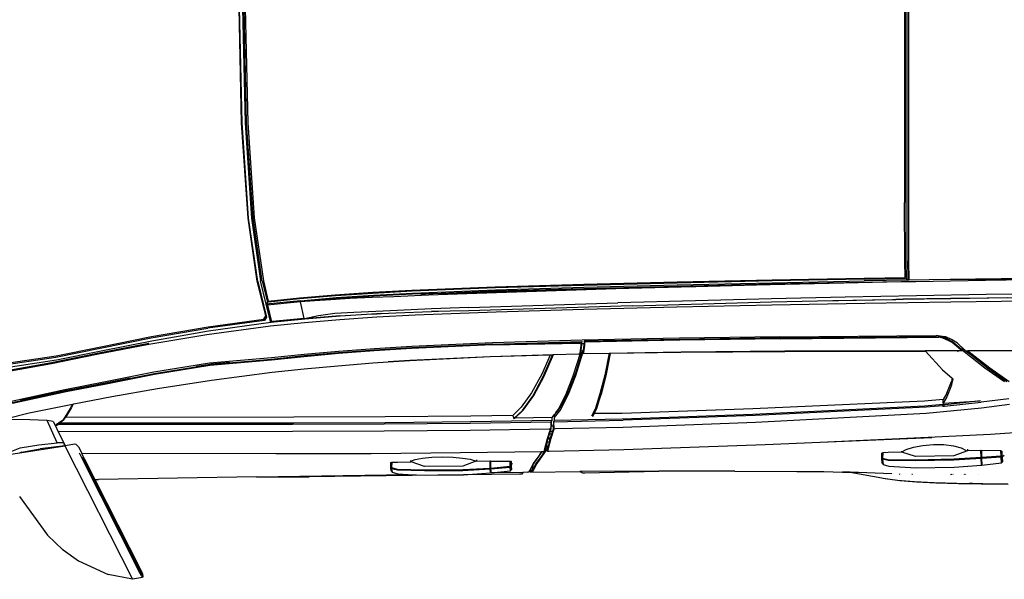
# Model space of a CAD drawing. Units: inches. Extents: x 22042254 to 25404563, y 17568978 to 17626777.
# Tile 14 of 45: x 22042341.458 to 22042342.604, y 17568977.553 to 17568978.204. Entities that reach past the tile are written whole.
import ezdxf

# ---------------------------------------------------------------- set-up
doc = ezdxf.new("R2010")
doc.units = ezdxf.units.IN
doc.header["$MEASUREMENT"] = 0
doc.layers.add('A-SITE-VEHI', color=8, linetype='Continuous', lineweight=18)
doc.layers.add('Edges', color=250, linetype='Continuous')

# ---------------------------------------------------------------- blocks, each defined once
blk = doc.blocks.new('Nissan Qashqai pl')
at = {"layer": 'Edges'}
for p, q in [((8.8918, 12.7444), (9.0186, 12.9956)), ((9.0186, 12.9956), (8.9731, 12.9865)), ((9.0374, 12.9925), (9.0186, 12.9956)), ((8.9173, 12.961), (8.9731, 12.9865)), ((9.0333, 12.9845), (8.9232, 12.7662)), ((9.0386, 12.9907), (8.9254, 12.7664)), ((8.9483, 12.8082), (9.0343, 12.9785)), ((9.0356, 12.9888), (9.0333, 12.9845)), ((9.0343, 12.9785), (9.0347, 12.9794)), ((9.0347, 12.9794), (9.0362, 12.9822)), ((9.0356, 12.9888), (9.0374, 12.9925)), ((9.0362, 12.9822), (9.037, 12.9838)), ((9.0371, 12.9841), (9.037, 12.9838)), ((9.0371, 12.9841), (9.0376, 12.985)), ((9.0376, 12.985), (9.0371, 12.9847)), ((9.0386, 12.9907), (9.0374, 12.9925)), ((9.0376, 12.985), (9.0386, 12.9907)), ((8.8885, 12.9405), (8.9173, 12.961)), ((8.8591, 12.9127), (8.8879, 12.94)), ((8.8885, 12.9405), (8.8879, 12.94)), ((8.8066, 12.84), (8.8591, 12.9127)), ((10.4573, 12.8093), (10.4889, 12.8119)), ((10.4613, 12.8099), (10.4926, 12.8125)), ((10.4889, 12.8119), (10.526, 12.8138)), ((10.4926, 12.8125), (10.5294, 12.8143)), ((10.526, 12.8138), (10.569, 12.8151)), ((10.5294, 12.8143), (10.5719, 12.8156)), ((10.569, 12.8151), (10.5919, 12.8155)), ((10.5719, 12.8156), (10.6176, 12.8164)), ((10.5919, 12.8155), (10.6151, 12.8159)), ((10.5981, 12.8157), (10.5919, 12.8155)), ((10.6174, 12.816), (10.5981, 12.8157)), ((10.6151, 12.8159), (10.6644, 12.8162)), ((10.6176, 12.8164), (10.6651, 12.8167)), ((8.928, 12.7679), (8.9483, 12.8082)), ((8.9483, 12.8082), (8.9552, 12.8081)), ((9.2517, 12.8031), (8.9552, 12.8081)), ((9.2517, 12.8031), (9.351, 12.803)), ((9.2517, 12.8031), (9.5372, 12.7983)), ((9.641, 12.7991), (9.351, 12.803)), ((9.5052, 12.7918), (9.5044, 12.7856)), ((9.5052, 12.7918), (9.5069, 12.7941)), ((9.5061, 12.7878), (9.5069, 12.7941)), ((9.5069, 12.7941), (9.5176, 12.7972)), ((9.5679, 12.792), (9.5168, 12.7904)), ((9.5176, 12.7972), (9.5372, 12.7983)), ((9.5372, 12.7983), (9.5689, 12.7999)), ((9.6401, 12.7914), (9.5679, 12.792)), ((9.5689, 12.7999), (9.641, 12.7991)), ((9.641, 12.7991), (9.6921, 12.7956)), ((9.7466, 12.7978), (9.641, 12.7991)), ((9.692, 12.7943), (9.6913, 12.7886)), ((9.6921, 12.7956), (9.692, 12.7943)), ((9.6922, 12.7943), (9.692, 12.7943)), ((9.6922, 12.7943), (9.6921, 12.7956)), ((9.7526, 12.7946), (9.6921, 12.7956)), ((9.6922, 12.7885), (9.693, 12.7955)), ((9.6922, 12.7885), (9.6922, 12.7943)), ((9.693, 12.7955), (9.7296, 12.7914)), ((9.7511, 12.7979), (9.7466, 12.7978)), ((9.7526, 12.7946), (9.7511, 12.7979)), ((9.7623, 12.7945), (9.7526, 12.7946)), ((9.7623, 12.7945), (9.7643, 12.7937)), ((9.7643, 12.7937), (9.7652, 12.7927)), ((9.7643, 12.7937), (9.7648, 12.7929)), ((9.7648, 12.7929), (9.7648, 12.7929)), ((9.7648, 12.7929), (9.7664, 12.7902)), ((9.7652, 12.7927), (9.7665, 12.7907)), ((9.7667, 12.7933), (9.7665, 12.7907)), ((9.7677, 12.7944), (9.7667, 12.7933)), ((9.7676, 12.7931), (9.7667, 12.7933)), ((9.7673, 12.7899), (9.7676, 12.7931)), ((9.769, 12.7926), (9.7676, 12.7931)), ((9.7677, 12.7944), (9.7677, 12.7944)), ((9.77, 12.7936), (9.7677, 12.7944)), ((9.7677, 12.7944), (9.8598, 12.7928)), ((9.7712, 12.7892), (9.769, 12.7926)), ((9.7734, 12.7884), (9.77, 12.7936)), ((9.8598, 12.7928), (9.8614, 12.7937)), ((9.8643, 12.7927), (9.8598, 12.7928)), ((9.8614, 12.7937), (9.8647, 12.7956)), ((10.0085, 12.7922), (9.8643, 12.7927)), ((9.8647, 12.7956), (9.869, 12.7954)), ((9.869, 12.7954), (10.0085, 12.7922)), ((10.0124, 12.7922), (10.0085, 12.7922)), ((10.1513, 12.7924), (10.0124, 12.7922)), ((10.1513, 12.7924), (10.2677, 12.793)), ((10.2677, 12.793), (10.3189, 12.7931)), ((10.3189, 12.7931), (10.3537, 12.7939)), ((10.3537, 12.7939), (10.3832, 12.7945)), ((10.3679, 12.7944), (10.3537, 12.7939)), ((10.3679, 12.7944), (10.4275, 12.8051)), ((10.4468, 12.7976), (10.3679, 12.7944)), ((10.4275, 12.8051), (10.4304, 12.8056)), ((10.4304, 12.8056), (10.4339, 12.8061)), ((10.4339, 12.8061), (10.4573, 12.8093)), ((10.4339, 12.8061), (10.4345, 12.8062)), ((10.4345, 12.8062), (10.4613, 12.8099)), ((10.4503, 12.7976), (10.4502, 12.7976)), ((10.4603, 12.7976), (10.4613, 12.7978)), ((10.4838, 12.7977), (10.4852, 12.7982)), ((10.5565, 12.7985), (10.5591, 12.7977)), ((10.5615, 12.7978), (10.5617, 12.7985)), ((10.583, 12.7984), (10.5834, 12.798)), ((10.5836, 12.798), (10.5831, 12.7984)), ((10.5847, 12.798), (10.5841, 12.7984)), ((10.5873, 12.7981), (10.5873, 12.7981)), ((10.6087, 12.7983), (10.6087, 12.7984)), ((9.5037, 12.7806), (9.5045, 12.7814)), ((9.5044, 12.7856), (9.5045, 12.7814)), ((9.5045, 12.7814), (9.5045, 12.7759)), ((9.5045, 12.7759), (9.5063, 12.7755)), ((9.5168, 12.7904), (9.5061, 12.7878)), ((9.5061, 12.7856), (9.5167, 12.7883)), ((9.5063, 12.7755), (9.5061, 12.7856)), ((9.5063, 12.7755), (9.5168, 12.7751)), ((9.5167, 12.7883), (9.5679, 12.7899)), ((9.5168, 12.7751), (9.5423, 12.7746)), ((9.5423, 12.7746), (9.5422, 12.7736)), ((9.5422, 12.7736), (9.5422, 12.7725)), ((9.5422, 12.7736), (9.5424, 12.7735)), ((9.5426, 12.7747), (9.5423, 12.7746)), ((9.5426, 12.7747), (9.5424, 12.7735)), ((9.5424, 12.7735), (9.5503, 12.7706)), ((9.5678, 12.7837), (9.5426, 12.7747)), ((9.64, 12.7831), (9.5678, 12.7837)), ((9.5679, 12.7899), (9.64, 12.7892)), ((9.64, 12.7892), (9.6912, 12.7865)), ((9.6645, 12.7737), (9.64, 12.7831)), ((9.6913, 12.7886), (9.6401, 12.7914)), ((9.6633, 12.7726), (9.6645, 12.7737)), ((9.6655, 12.7733), (9.6645, 12.7737)), ((9.6655, 12.7733), (9.6911, 12.7732)), ((9.6655, 12.7713), (9.6655, 12.7733)), ((9.6912, 12.7811), (9.6911, 12.7796)), ((9.6911, 12.7796), (9.6911, 12.7732)), ((9.6913, 12.7886), (9.6912, 12.7865)), ((9.6912, 12.7865), (9.6912, 12.7811)), ((9.692, 12.7811), (9.6912, 12.7811)), ((9.692, 12.7811), (9.6921, 12.7864)), ((9.692, 12.7796), (9.692, 12.7811)), ((9.692, 12.7733), (9.692, 12.7796)), ((9.692, 12.7733), (9.7287, 12.7734)), ((9.6922, 12.7885), (9.6921, 12.7864)), ((9.6921, 12.7864), (9.7288, 12.7832)), ((9.7288, 12.7854), (9.6922, 12.7885)), ((9.7288, 12.7832), (9.7287, 12.7734)), ((9.7287, 12.7734), (9.7305, 12.7738)), ((9.7296, 12.7914), (9.7288, 12.7854)), ((9.7306, 12.7834), (9.7288, 12.7854)), ((9.7288, 12.7854), (9.7288, 12.7832)), ((9.7288, 12.7832), (9.7306, 12.7834)), ((9.7296, 12.7914), (9.7314, 12.7895)), ((9.7305, 12.7738), (9.7306, 12.7834)), ((9.7305, 12.7738), (9.7313, 12.7798)), ((9.7306, 12.7834), (9.7314, 12.7895)), ((9.7314, 12.7895), (9.7313, 12.7798)), ((9.733, 12.7782), (9.7313, 12.7798)), ((9.7665, 12.7904), (9.7664, 12.7902)), ((9.7664, 12.7902), (9.7674, 12.7885)), ((9.7665, 12.7907), (9.7676, 12.7889)), ((9.7673, 12.7897), (9.7673, 12.7899)), ((9.7673, 12.7897), (9.7676, 12.7889)), ((9.7674, 12.7885), (9.7728, 12.7781)), ((9.7676, 12.7889), (9.7684, 12.7875)), ((9.7676, 12.7887), (9.7678, 12.7882)), ((9.7684, 12.7875), (9.7717, 12.781)), ((9.7707, 12.7848), (9.7709, 12.7893)), ((9.7717, 12.781), (9.7707, 12.7848)), ((9.7709, 12.7893), (9.7712, 12.7892)), ((9.7724, 12.7874), (9.7712, 12.7892)), ((9.7717, 12.781), (9.7738, 12.7771)), ((9.7778, 12.777), (9.7724, 12.7874)), ((9.7728, 12.7781), (9.7832, 12.7637)), ((9.7788, 12.778), (9.7734, 12.7884)), ((9.7738, 12.7771), (9.7842, 12.7627)), ((9.7883, 12.7626), (9.7778, 12.777)), ((9.7894, 12.7636), (9.7788, 12.778)), ((10.4282, 12.7775), (10.4274, 12.7679)), ((10.4282, 12.7775), (10.4299, 12.7798)), ((10.4291, 12.77), (10.4299, 12.7798)), ((10.4299, 12.7798), (10.4406, 12.7829)), ((10.4406, 12.7829), (10.4919, 12.7858)), ((10.4919, 12.7858), (10.564, 12.7851)), ((10.564, 12.7851), (10.6151, 12.7813)), ((10.615, 12.7803), (10.6142, 12.7686)), ((10.6151, 12.7813), (10.615, 12.7803)), ((10.615, 12.7676), (10.6151, 12.7803)), ((10.6151, 12.7803), (10.615, 12.7803)), ((10.6151, 12.7803), (10.6151, 12.7813)), ((10.6151, 12.7685), (10.616, 12.7812)), ((10.616, 12.7812), (10.6526, 12.7768)), ((10.6526, 12.7768), (10.6518, 12.7657)), ((10.6526, 12.7768), (10.6543, 12.7749)), ((10.6537, 12.7658), (10.6543, 12.7749)), ((10.6543, 12.7749), (10.6543, 12.7656)), ((8.7858, 12.7613), (8.807, 12.758)), ((8.8102, 12.7568), (8.807, 12.758)), ((8.807, 12.758), (8.8918, 12.7444)), ((8.8102, 12.7568), (8.8455, 12.7506)), ((8.9171, 12.7464), (8.9233, 12.7586)), ((8.9232, 12.7662), (8.9194, 12.7588)), ((8.925, 12.762), (8.9233, 12.7586)), ((8.9233, 12.7586), (9.2886, 12.7594)), ((8.928, 12.7679), (8.925, 12.762)), ((9.2886, 12.7594), (9.4673, 12.7589)), ((9.4673, 12.7589), (9.6358, 12.7575)), ((9.5503, 12.7706), (9.5641, 12.7681)), ((9.5641, 12.7681), (9.5818, 12.766)), ((9.5818, 12.766), (9.6016, 12.7651)), ((9.6016, 12.7651), (9.6215, 12.766)), ((9.6215, 12.766), (9.6395, 12.7676)), ((9.6358, 12.7575), (9.7887, 12.7552)), ((9.6395, 12.7676), (9.654, 12.7697)), ((9.654, 12.7697), (9.6633, 12.7726)), ((9.6911, 12.7732), (9.692, 12.7733)), ((9.7832, 12.7637), (9.7887, 12.7552)), ((9.7842, 12.7627), (9.7891, 12.7552)), ((9.7933, 12.7549), (9.7883, 12.7626)), ((9.7887, 12.7552), (9.7891, 12.7552)), ((9.7891, 12.7552), (9.79, 12.7552)), ((9.7965, 12.7526), (9.7894, 12.7636)), ((9.79, 12.7552), (9.7931, 12.7552)), ((9.7931, 12.7552), (9.7934, 12.7535)), ((9.7931, 12.7552), (9.7933, 12.7549)), ((9.7933, 12.7549), (9.7941, 12.7541)), ((9.7993, 12.755), (9.7986, 12.7544)), ((9.7999, 12.7522), (9.7993, 12.755)), ((9.7993, 12.755), (9.8024, 12.7549)), ((9.8024, 12.7549), (9.9426, 12.7518)), ((10.4263, 12.7665), (10.4274, 12.7674)), ((10.4274, 12.7679), (10.4274, 12.7674)), ((10.4274, 12.7674), (10.4275, 12.7586)), ((10.4293, 12.7579), (10.4275, 12.7586)), ((10.4398, 12.7724), (10.4291, 12.77)), ((10.4291, 12.7677), (10.4398, 12.7701)), ((10.4293, 12.7579), (10.4291, 12.7677)), ((10.4398, 12.7573), (10.4293, 12.7579)), ((10.4909, 12.773), (10.4398, 12.7724)), ((10.4398, 12.7701), (10.4909, 12.7708)), ((10.4653, 12.7564), (10.4398, 12.7573)), ((10.4653, 12.7561), (10.4652, 12.7545)), ((10.4908, 12.7648), (10.4653, 12.7564)), ((10.4653, 12.7564), (10.4653, 12.7561)), ((10.4653, 12.7564), (10.4653, 12.7564)), ((10.4653, 12.7564), (10.4653, 12.7561)), ((10.4653, 12.7561), (10.4653, 12.7561)), ((10.4653, 12.7561), (10.4732, 12.7517)), ((10.563, 12.7633), (10.4908, 12.7648)), ((10.5631, 12.7715), (10.4909, 12.773)), ((10.4909, 12.7708), (10.563, 12.7692)), ((10.563, 12.7692), (10.6142, 12.7663)), ((10.5867, 12.7545), (10.563, 12.7633)), ((10.6142, 12.7686), (10.5631, 12.7715)), ((10.6142, 12.766), (10.6141, 12.7537)), ((10.6142, 12.7686), (10.6142, 12.7677)), ((10.6142, 12.7677), (10.615, 12.7676)), ((10.6142, 12.7677), (10.6142, 12.7663)), ((10.6142, 12.7663), (10.6142, 12.766)), ((10.6151, 12.7676), (10.615, 12.7676)), ((10.615, 12.7537), (10.6151, 12.7659)), ((10.6518, 12.7657), (10.6151, 12.7685)), ((10.6151, 12.7676), (10.6151, 12.7685)), ((10.6151, 12.7662), (10.6151, 12.7676)), ((10.6151, 12.7662), (10.6518, 12.7634)), ((10.6151, 12.7659), (10.6151, 12.7662)), ((10.6518, 12.7634), (10.6517, 12.754)), ((10.6536, 12.7639), (10.6518, 12.7657)), ((10.6518, 12.7657), (10.6518, 12.7634)), ((10.6518, 12.7634), (10.6536, 12.7639)), ((10.6543, 12.7656), (10.6535, 12.7546)), ((10.6535, 12.7546), (10.6536, 12.7639)), ((10.6536, 12.7639), (10.6537, 12.7658)), ((10.6537, 12.7658), (10.6543, 12.7656)), ((10.6578, 12.7628), (10.6543, 12.7656)), ((8.7917, 12.7547), (8.8075, 12.7486)), ((8.8075, 12.7486), (8.8429, 12.7426)), ((8.8429, 12.7426), (8.8771, 12.7388)), ((8.8918, 12.7444), (8.8455, 12.7506)), ((8.8771, 12.7388), (8.8585, 12.6969)), ((8.8895, 12.7393), (8.8771, 12.7388)), ((8.8815, 12.7228), (8.892, 12.7444)), ((8.8815, 12.7228), (8.8895, 12.7393)), ((8.8908, 12.7421), (8.8895, 12.7393)), ((8.8906, 12.7418), (8.8895, 12.7393)), ((8.8906, 12.7418), (8.8911, 12.7428)), ((8.892, 12.7444), (8.8908, 12.7421)), ((8.8911, 12.7428), (8.8919, 12.7444)), ((8.8911, 12.7428), (8.8919, 12.7444)), ((8.8919, 12.7444), (8.8911, 12.7428)), ((8.8919, 12.7444), (8.8918, 12.7444)), ((8.892, 12.7444), (8.8919, 12.7444)), ((8.8919, 12.7444), (8.8919, 12.7444)), ((8.8919, 12.7444), (8.8919, 12.7444)), ((8.9106, 12.7413), (8.892, 12.7444)), ((8.892, 12.7444), (8.892, 12.7444)), ((8.9131, 12.7421), (8.9106, 12.7413)), ((8.9171, 12.7464), (8.9131, 12.7421)), ((8.9171, 12.7464), (8.917, 12.7468)), ((9.7934, 12.7535), (9.7938, 12.7538)), ((9.7934, 12.7535), (9.7937, 12.7524)), ((9.7937, 12.7524), (9.7992, 12.7308)), ((9.7941, 12.7541), (9.7943, 12.7535)), ((9.7955, 12.7516), (9.7943, 12.7535)), ((9.7943, 12.7535), (9.7964, 12.7453)), ((9.7963, 12.7523), (9.7955, 12.7516)), ((9.7963, 12.7523), (9.7963, 12.7524)), ((9.7964, 12.7524), (9.7963, 12.7523)), ((9.7992, 12.7476), (9.7963, 12.7523)), ((9.7967, 12.7526), (9.7964, 12.7524)), ((9.7964, 12.7525), (9.7964, 12.7524)), ((9.7964, 12.7524), (9.7996, 12.7475)), ((9.7964, 12.7453), (9.7992, 12.7476)), ((9.7964, 12.7453), (9.7973, 12.7418)), ((9.7983, 12.7541), (9.7965, 12.7526)), ((9.7965, 12.7526), (9.7967, 12.7526)), ((9.7977, 12.7535), (9.7967, 12.7526)), ((9.7967, 12.7526), (9.7986, 12.7526)), ((9.7977, 12.7431), (9.7973, 12.7418)), ((9.7973, 12.7418), (9.7977, 12.7409)), ((9.7973, 12.7418), (9.7977, 12.7399)), ((9.7982, 12.754), (9.7977, 12.7535)), ((9.7977, 12.7444), (9.7985, 12.7451)), ((9.7985, 12.7451), (9.7977, 12.7431)), ((9.7977, 12.7431), (9.7977, 12.7444)), ((9.7977, 12.7399), (9.7977, 12.7409)), ((9.7977, 12.7409), (9.7987, 12.7388)), ((9.7977, 12.7399), (9.7978, 12.7397)), ((9.7987, 12.7388), (9.7978, 12.7397)), ((9.7978, 12.7397), (9.7987, 12.7362)), ((9.7983, 12.7541), (9.7982, 12.754)), ((9.7986, 12.7526), (9.7982, 12.754)), ((9.7986, 12.7544), (9.7983, 12.7541)), ((9.7989, 12.7461), (9.7985, 12.7451)), ((9.7988, 12.7516), (9.7986, 12.7526)), ((9.7987, 12.7388), (9.7992, 12.7377)), ((9.7987, 12.7362), (9.7992, 12.7377)), ((9.7998, 12.7477), (9.7988, 12.7516)), ((9.7998, 12.7466), (9.7989, 12.7461)), ((9.7998, 12.7466), (9.7992, 12.7476)), ((9.7992, 12.7377), (9.8027, 12.7364)), ((9.7996, 12.7475), (9.7998, 12.7477)), ((9.8002, 12.7461), (9.7996, 12.7475)), ((9.8001, 12.7468), (9.7996, 12.7475)), ((9.8001, 12.7468), (9.7998, 12.7477)), ((9.8003, 12.7458), (9.7998, 12.7466)), ((9.8054, 12.7307), (9.7999, 12.7522)), ((9.8002, 12.7461), (9.8001, 12.7468)), ((9.8003, 12.7458), (9.8002, 12.7461)), ((9.8027, 12.7364), (9.8003, 12.7458)), ((9.8031, 12.7349), (9.8027, 12.7364)), ((9.9426, 12.7518), (10.2081, 12.7424)), ((10.2081, 12.7424), (10.312, 12.7377)), ((10.312, 12.7377), (10.5214, 12.7293)), ((10.312, 12.7377), (10.5147, 12.7285)), ((10.4732, 12.7517), (10.4871, 12.7474)), ((10.4871, 12.7474), (10.5048, 12.744)), ((10.5048, 12.744), (10.5246, 12.7423)), ((10.5246, 12.7423), (10.5445, 12.7425)), ((10.5445, 12.7425), (10.5625, 12.7446)), ((10.5625, 12.7446), (10.5769, 12.7484)), ((10.5769, 12.7484), (10.5863, 12.7537)), ((10.5863, 12.7537), (10.5867, 12.7545)), ((10.5885, 12.7538), (10.5867, 12.7545)), ((10.5885, 12.751), (10.5885, 12.7538)), ((10.6141, 12.7537), (10.5885, 12.7538)), ((10.6141, 12.7537), (10.615, 12.7537)), ((10.6517, 12.754), (10.615, 12.7537)), ((10.6535, 12.7546), (10.6517, 12.754)), ((8.8734, 12.7057), (8.8793, 12.7181)), ((8.8793, 12.7181), (8.8815, 12.7228)), ((9.3194, 12.7179), (8.8793, 12.7181)), ((9.4919, 12.7173), (9.3194, 12.7179)), ((9.7987, 12.7362), (9.8002, 12.7301)), ((9.7992, 12.7308), (9.8044, 12.7151)), ((9.8002, 12.7301), (9.8008, 12.7285)), ((9.8008, 12.7285), (9.8014, 12.7303)), ((9.8008, 12.7285), (9.8014, 12.7265)), ((9.8014, 12.7303), (9.8031, 12.7349)), ((9.8043, 12.7303), (9.8014, 12.7303)), ((9.8014, 12.7265), (9.803, 12.723)), ((9.8014, 12.7265), (9.8026, 12.723)), ((9.803, 12.723), (9.8026, 12.723)), ((9.8026, 12.723), (9.8046, 12.7171)), ((9.8067, 12.7229), (9.803, 12.723)), ((9.8043, 12.7303), (9.8031, 12.7349)), ((9.8044, 12.73), (9.8043, 12.7303)), ((9.8067, 12.7229), (9.8044, 12.73)), ((9.8106, 12.715), (9.8054, 12.7307)), ((9.8086, 12.7171), (9.8067, 12.7229)), ((10.5147, 12.7285), (10.6318, 12.7228)), ((10.6318, 12.7228), (10.6955, 12.7184)), ((8.87, 12.6987), (8.8734, 12.7057)), ((8.8734, 12.7057), (8.8768, 12.7057)), ((8.8751, 12.7054), (8.8768, 12.7057)), ((8.8893, 12.6956), (8.8751, 12.7054)), ((8.8768, 12.7057), (8.879, 12.704)), ((8.879, 12.704), (9.3198, 12.7039)), ((8.879, 12.704), (8.881, 12.7023)), ((9.3225, 12.7021), (8.881, 12.7023)), ((8.881, 12.7023), (8.8893, 12.6956)), ((9.3198, 12.7039), (9.4922, 12.7033)), ((9.4936, 12.7013), (9.3225, 12.7021)), ((9.6538, 12.7157), (9.4919, 12.7173)), ((9.4922, 12.7033), (9.654, 12.7018)), ((9.6552, 12.6997), (9.4936, 12.7013)), ((9.802, 12.7133), (9.6538, 12.7157)), ((9.654, 12.7018), (9.8061, 12.6994)), ((9.8078, 12.6971), (9.6552, 12.6997)), ((9.8051, 12.7132), (9.802, 12.7133)), ((9.8044, 12.7151), (9.8051, 12.7132)), ((9.8046, 12.7171), (9.8086, 12.7171)), ((9.8046, 12.7171), (9.8055, 12.7143)), ((9.8061, 12.6994), (9.8051, 12.7132)), ((9.8055, 12.7143), (9.8058, 12.7073)), ((9.8058, 12.7073), (9.8098, 12.7073)), ((9.8058, 12.7073), (9.8061, 12.6994)), ((9.8061, 12.6994), (9.8078, 12.6971)), ((9.8096, 12.7142), (9.8086, 12.7171)), ((9.8098, 12.7073), (9.8096, 12.7142)), ((9.8101, 12.6993), (9.8098, 12.7073)), ((9.8101, 12.6993), (9.8112, 12.7131)), ((9.8119, 12.697), (9.8101, 12.6993)), ((9.8101, 12.6993), (9.9411, 12.6966)), ((9.8112, 12.7131), (9.8106, 12.715)), ((9.8143, 12.713), (9.8112, 12.7131)), ((9.9414, 12.71), (9.8143, 12.713)), ((10.19, 12.7008), (9.9414, 12.71)), ((10.5113, 12.6839), (10.19, 12.7008)), ((8.7828, 12.6934), (8.8245, 12.6828)), ((8.8259, 12.6959), (8.7916, 12.6954)), ((8.8245, 12.6828), (8.9063, 12.6663)), ((8.8585, 12.6969), (8.8259, 12.6959)), ((8.87, 12.6987), (8.8585, 12.6969)), ((8.8893, 12.6956), (8.9021, 12.6745)), ((8.8913, 12.6936), (8.8893, 12.6956)), ((8.8927, 12.6913), (8.8913, 12.6936)), ((9.3224, 12.6911), (8.8927, 12.6913)), ((8.9041, 12.6725), (8.8927, 12.6913)), ((9.3225, 12.6911), (9.3224, 12.6911)), ((9.4936, 12.6904), (9.3225, 12.6911)), ((9.6552, 12.6888), (9.4936, 12.6904)), ((9.7337, 12.6875), (9.6552, 12.6888)), ((9.7337, 12.6875), (9.7357, 12.6935)), ((9.7499, 12.6721), (9.7337, 12.6875)), ((9.7357, 12.6935), (9.7378, 12.6924)), ((9.7357, 12.6935), (9.7519, 12.678)), ((9.7378, 12.6924), (9.754, 12.677)), ((9.8078, 12.6913), (9.7378, 12.6924)), ((9.8078, 12.6971), (9.8078, 12.6913)), ((9.8078, 12.6913), (9.8119, 12.6862)), ((9.9393, 12.6944), (9.8119, 12.697)), ((9.8119, 12.6912), (9.8119, 12.697)), ((9.8241, 12.6756), (9.8119, 12.6912)), ((9.8119, 12.6862), (9.8119, 12.6912)), ((9.8147, 12.6826), (9.8119, 12.6862)), ((9.8147, 12.6826), (9.8147, 12.6826)), ((9.8147, 12.6826), (9.8201, 12.6756)), ((9.8241, 12.6706), (9.8147, 12.6826)), ((9.8891, 12.6741), (9.8818, 12.6891)), ((9.8867, 12.6842), (9.8838, 12.6901)), ((9.9393, 12.684), (9.8867, 12.6842)), ((9.8911, 12.675), (9.8867, 12.6842)), ((10.1849, 12.6857), (9.9393, 12.6944)), ((10.1849, 12.6754), (9.9393, 12.684)), ((10.1894, 12.6879), (9.9411, 12.6966)), ((10.5079, 12.6703), (10.1849, 12.6857)), ((10.5109, 12.6721), (10.1894, 12.6879)), ((10.6152, 12.674), (10.5113, 12.6839)), ((8.8941, 12.6418), (8.7925, 12.664)), ((8.8942, 12.6432), (8.7931, 12.6653)), ((8.9021, 12.6745), (8.9063, 12.6663)), ((8.9075, 12.6661), (8.9041, 12.6725)), ((8.9063, 12.6663), (8.9075, 12.6661)), ((8.9075, 12.6661), (8.9087, 12.6658)), ((8.9087, 12.6658), (8.9797, 12.6518)), ((9.7692, 12.6453), (9.7499, 12.6721)), ((9.7519, 12.678), (9.7713, 12.6512)), ((9.754, 12.677), (9.7733, 12.6502)), ((9.8201, 12.6756), (9.8338, 12.6486)), ((9.8378, 12.6485), (9.8241, 12.6756)), ((9.8378, 12.6435), (9.8241, 12.6706)), ((9.8978, 12.6472), (9.8891, 12.6741)), ((9.8911, 12.6749), (9.8911, 12.675)), ((9.8931, 12.6691), (9.8911, 12.6749)), ((9.8911, 12.6749), (9.8998, 12.6481)), ((9.8931, 12.669), (9.8931, 12.6691)), ((9.8931, 12.669), (9.9018, 12.6421)), ((10.5079, 12.6607), (10.1849, 12.6754)), ((10.543, 12.6671), (10.5079, 12.6703)), ((10.5417, 12.6693), (10.5109, 12.6721)), ((10.5417, 12.6693), (10.5427, 12.6702)), ((10.5417, 12.6693), (10.543, 12.6671)), ((10.5436, 12.6687), (10.5427, 12.6702)), ((10.5427, 12.6702), (10.5458, 12.67)), ((10.544, 12.6678), (10.543, 12.6671)), ((10.543, 12.6646), (10.543, 12.6671)), ((10.543, 12.6646), (10.543, 12.6576)), ((10.5439, 12.6646), (10.543, 12.6646)), ((10.5502, 12.6526), (10.543, 12.6646)), ((10.544, 12.6678), (10.5436, 12.6687)), ((10.5439, 12.6646), (10.613, 12.6601)), ((10.547, 12.6674), (10.544, 12.6678)), ((10.5458, 12.67), (10.6144, 12.6629)), ((10.613, 12.6601), (10.547, 12.6674)), ((10.6664, 12.6566), (10.6144, 12.6629)), ((10.6678, 12.6672), (10.6152, 12.674)), ((8.8918, 12.6392), (8.7881, 12.6621)), ((8.8083, 12.6591), (8.8954, 12.6403)), ((8.9797, 12.6518), (9.0656, 12.6372)), ((9.7885, 12.6099), (9.7692, 12.6453)), ((9.7713, 12.6512), (9.7905, 12.6158)), ((9.7733, 12.6502), (9.7925, 12.6148)), ((9.8338, 12.6486), (9.8475, 12.613)), ((9.8516, 12.6129), (9.8378, 12.6485)), ((9.9066, 12.6119), (9.8978, 12.6472)), ((9.9086, 12.6129), (9.8998, 12.6481)), ((10.543, 12.6576), (10.5079, 12.6607)), ((10.5502, 12.6456), (10.543, 12.6576)), ((10.5584, 12.6306), (10.5502, 12.6526)), ((10.5502, 12.6456), (10.5584, 12.6236)), ((8.9679, 12.6241), (8.8918, 12.6392)), ((9.0601, 12.6092), (8.8941, 12.6418)), ((8.9696, 12.6285), (8.8942, 12.6432)), ((8.8961, 12.6401), (8.9704, 12.6257)), ((9.06, 12.6106), (8.9696, 12.6285)), ((8.9704, 12.6257), (8.9708, 12.6256)), ((8.9708, 12.6256), (9.0143, 12.6169)), ((9.0656, 12.6372), (9.1676, 12.6212)), ((9.8516, 12.6079), (9.8378, 12.6435)), ((9.9018, 12.6421), (9.9106, 12.6068)), ((10.5584, 12.6306), (10.5617, 12.619)), ((8.8666, 12.5888), (8.7287, 12.6134)), ((8.7292, 12.6146), (8.8666, 12.5901)), ((9.0591, 12.6065), (8.9679, 12.6241)), ((9.1644, 12.5938), (9.06, 12.6106)), ((9.1645, 12.5924), (9.0601, 12.6092)), ((9.1676, 12.6212), (9.2814, 12.6065)), ((9.8039, 12.5741), (9.7885, 12.6099)), ((9.7905, 12.6158), (9.8087, 12.574)), ((9.7925, 12.6148), (9.8107, 12.573)), ((9.8475, 12.613), (9.8611, 12.5708)), ((9.8652, 12.5704), (9.8516, 12.6129)), ((9.8652, 12.5654), (9.8516, 12.6079)), ((9.9149, 12.5705), (9.9066, 12.6119)), ((9.9169, 12.5714), (9.9086, 12.6129)), ((9.9106, 12.6068), (9.9177, 12.5714)), ((10.5419, 12.6018), (10.56, 12.6176)), ((10.56, 12.6176), (10.5584, 12.6236)), ((10.56, 12.6176), (10.5617, 12.619)), ((10.6583, 12.6245), (10.6215, 12.5986)), ((10.6627, 12.6241), (10.6261, 12.5984)), ((10.6306, 12.5982), (10.6671, 12.6238)), ((8.7481, 12.5968), (8.8745, 12.5782)), ((8.7491, 12.594), (8.8754, 12.5755)), ((8.8761, 12.5839), (8.7496, 12.6025)), ((8.8666, 12.5901), (8.9521, 12.5726)), ((8.9522, 12.5713), (8.8666, 12.5888)), ((9.1639, 12.5895), (9.0591, 12.6065)), ((9.1393, 12.5951), (9.1647, 12.591)), ((9.2801, 12.5794), (9.1639, 12.5895)), ((9.2803, 12.5836), (9.1644, 12.5938)), ((9.2804, 12.5821), (9.1645, 12.5924)), ((9.1647, 12.591), (9.1668, 12.5908)), ((9.1668, 12.5908), (9.2019, 12.5877)), ((9.2814, 12.6065), (9.3416, 12.5999)), ((9.3416, 12.5999), (9.4048, 12.5941)), ((9.4048, 12.5941), (9.471, 12.5888)), ((9.471, 12.5888), (9.4997, 12.5869)), ((10.51, 12.5666), (10.5419, 12.6018)), ((10.6215, 12.5986), (10.5796, 12.5655)), ((10.5892, 12.5659), (10.6306, 12.5982)), ((10.6261, 12.5984), (10.593, 12.5726)), ((8.8745, 12.5782), (8.9583, 12.5609)), ((8.8754, 12.5755), (8.9591, 12.5583)), ((8.9598, 12.5666), (8.8761, 12.5839)), ((8.9521, 12.5726), (9.0495, 12.5536)), ((9.0497, 12.5523), (8.9522, 12.5713)), ((9.3418, 12.5729), (9.2801, 12.5794)), ((9.3418, 12.5771), (9.2803, 12.5836)), ((9.3419, 12.5756), (9.2804, 12.5821)), ((9.4062, 12.5713), (9.3418, 12.5771)), ((9.4064, 12.5671), (9.3418, 12.5729)), ((9.4063, 12.5699), (9.3419, 12.5756)), ((9.4735, 12.5663), (9.4062, 12.5713)), ((9.4736, 12.5648), (9.4063, 12.5699)), ((9.5404, 12.5844), (9.4997, 12.5869)), ((9.4997, 12.5869), (9.5403, 12.5842)), ((9.5403, 12.5842), (9.6913, 12.5767)), ((9.6912, 12.5774), (9.5404, 12.5844)), ((9.8039, 12.5741), (9.6912, 12.5774)), ((9.6913, 12.5767), (9.8099, 12.573)), ((9.8087, 12.574), (9.8039, 12.5741)), ((9.8099, 12.573), (9.8087, 12.574)), ((9.8099, 12.573), (9.8107, 12.573)), ((9.8107, 12.573), (9.8573, 12.5716)), ((9.8573, 12.5716), (9.8603, 12.5715)), ((9.8603, 12.5715), (9.8605, 12.5696)), ((9.8611, 12.5708), (9.8603, 12.5715)), ((9.8612, 12.5707), (9.8611, 12.5708)), ((9.8612, 12.5707), (9.8615, 12.5688)), ((9.8652, 12.5706), (9.8664, 12.5714)), ((9.8652, 12.5706), (9.8665, 12.5695)), ((9.8652, 12.5704), (9.8652, 12.5706)), ((9.8652, 12.5704), (9.8652, 12.5704)), ((9.8652, 12.5704), (9.8652, 12.5654)), ((9.8655, 12.5687), (9.8652, 12.5704)), ((9.8665, 12.5695), (9.8664, 12.5714)), ((9.8664, 12.5714), (9.9149, 12.5705)), ((9.9149, 12.5705), (10.0505, 12.5681)), ((9.9177, 12.5714), (9.9169, 12.5714)), ((10.0501, 12.5695), (9.9177, 12.5714)), ((10.593, 12.5726), (10.584, 12.5655)), ((8.9583, 12.5609), (9.0538, 12.5419)), ((8.9591, 12.5583), (9.0546, 12.5394)), ((9.0552, 12.5477), (8.9598, 12.5666)), ((9.0495, 12.5536), (9.1584, 12.5351)), ((9.4739, 12.5621), (9.4064, 12.5671)), ((9.5437, 12.5619), (9.4735, 12.5663)), ((9.5438, 12.5605), (9.4736, 12.5648)), ((9.5443, 12.5579), (9.4739, 12.5621)), ((9.6953, 12.5549), (9.5437, 12.5619)), ((9.6954, 12.5535), (9.5438, 12.5605)), ((9.696, 12.551), (9.5443, 12.5579)), ((9.6953, 12.5549), (9.8598, 12.5517)), ((9.6953, 12.5549), (9.863, 12.5497)), ((9.6954, 12.5535), (9.8641, 12.5483)), ((9.8629, 12.5516), (9.8598, 12.5517)), ((9.8605, 12.5696), (9.8626, 12.5564)), ((9.8615, 12.5688), (9.8635, 12.5556)), ((9.8626, 12.5564), (9.8627, 12.5532)), ((9.8637, 12.5532), (9.8627, 12.5532)), ((9.8627, 12.5532), (9.8629, 12.5516)), ((9.8629, 12.5516), (9.863, 12.5497)), ((9.8635, 12.5556), (9.8637, 12.5532)), ((9.8643, 12.5532), (9.8637, 12.5532)), ((9.8637, 12.5532), (9.8638, 12.5508)), ((9.8677, 12.5531), (9.8643, 12.5532)), ((9.8675, 12.5555), (9.8655, 12.5687)), ((9.8686, 12.5562), (9.8665, 12.5695)), ((9.8677, 12.5531), (9.8675, 12.5555)), ((9.8678, 12.5507), (9.8677, 12.5531)), ((9.8689, 12.5515), (9.8686, 12.5562)), ((9.869, 12.5496), (9.8689, 12.5515)), ((10.2453, 12.568), (10.0501, 12.5695)), ((10.0505, 12.5681), (10.2453, 12.5664)), ((10.4292, 12.5674), (10.2453, 12.568)), ((10.2453, 12.5664), (10.4289, 12.5658)), ((10.4289, 12.5658), (10.5092, 12.5658)), ((10.5099, 12.5674), (10.4292, 12.5674)), ((10.5099, 12.5674), (10.5092, 12.5658)), ((10.5092, 12.5658), (10.5094, 12.5658)), ((10.5094, 12.5658), (10.51, 12.5666)), ((10.5783, 12.5659), (10.5094, 12.5658)), ((10.51, 12.5666), (10.5099, 12.5674)), ((10.57, 12.5517), (10.5589, 12.5451)), ((10.5764, 12.5642), (10.5598, 12.5507)), ((10.5776, 12.5633), (10.5612, 12.5498)), ((10.5834, 12.5641), (10.57, 12.5517)), ((10.57, 12.5517), (10.5821, 12.5633)), ((10.5709, 12.5675), (10.5705, 12.5671)), ((10.5719, 12.5682), (10.5709, 12.5675)), ((10.5783, 12.5659), (10.5764, 12.5642)), ((10.5776, 12.5633), (10.5783, 12.5659)), ((10.5796, 12.5655), (10.5776, 12.5633)), ((10.5796, 12.5655), (10.5783, 12.5659)), ((10.5796, 12.562), (10.5796, 12.5655)), ((10.5838, 12.5653), (10.5821, 12.5633)), ((10.584, 12.5647), (10.5834, 12.5641)), ((10.584, 12.5655), (10.5838, 12.5653)), ((10.584, 12.5655), (10.5841, 12.5655)), ((10.584, 12.5654), (10.584, 12.5655)), ((10.5847, 12.5655), (10.584, 12.5647)), ((10.584, 12.5647), (10.584, 12.5654)), ((10.5851, 12.5659), (10.5841, 12.5655)), ((10.5841, 12.5655), (10.5847, 12.5655)), ((10.5851, 12.5659), (10.5847, 12.5655)), ((10.5851, 12.5659), (10.5892, 12.5659)), ((10.6988, 12.5662), (10.5892, 12.5659)), ((9.0538, 12.5419), (9.1605, 12.5233)), ((9.0546, 12.5394), (9.1612, 12.5208)), ((9.1617, 12.5292), (9.0552, 12.5477)), ((9.1584, 12.5351), (9.2783, 12.5191)), ((9.8644, 12.5459), (9.696, 12.551)), ((9.8641, 12.5483), (9.863, 12.5497)), ((9.8638, 12.5508), (9.8641, 12.5483)), ((10.0472, 12.5423), (9.8644, 12.5459)), ((9.8681, 12.5482), (9.8678, 12.5507)), ((9.8681, 12.5482), (9.869, 12.5496)), ((10.0476, 12.5445), (9.8681, 12.5482)), ((10.0477, 12.5459), (9.869, 12.5496)), ((10.2357, 12.5398), (10.0472, 12.5423)), ((10.2367, 12.5419), (10.0476, 12.5445)), ((10.2369, 12.5433), (10.0477, 12.5459)), ((10.2357, 12.5398), (10.53, 12.5373)), ((10.2367, 12.5419), (10.5351, 12.5392)), ((10.2369, 12.5433), (10.5348, 12.5406)), ((10.4153, 12.5384), (10.4176, 12.5384)), ((10.4176, 12.5384), (10.4181, 12.5384)), ((10.4181, 12.5384), (10.4552, 12.538)), ((10.4181, 12.5384), (10.4181, 12.5384)), ((10.4778, 12.5378), (10.53, 12.5373)), ((10.5301, 12.5373), (10.53, 12.5373)), ((10.5335, 12.5378), (10.5301, 12.5373)), ((10.5419, 12.5391), (10.5335, 12.5378)), ((10.5422, 12.542), (10.5348, 12.5406)), ((10.5418, 12.5405), (10.5351, 12.5392)), ((10.5424, 12.5406), (10.5418, 12.5405)), ((10.5419, 12.5391), (10.5463, 12.541)), ((10.5479, 12.54), (10.5419, 12.5391)), ((10.5522, 12.5465), (10.5422, 12.542)), ((10.5495, 12.5438), (10.5424, 12.5406)), ((10.5463, 12.541), (10.5551, 12.5457)), ((10.5589, 12.5451), (10.5479, 12.54)), ((10.5546, 12.546), (10.5495, 12.5438)), ((10.5598, 12.5507), (10.5522, 12.5465)), ((10.5583, 12.5481), (10.5546, 12.546)), ((10.5551, 12.5457), (10.5583, 12.5481)), ((10.5612, 12.5498), (10.5583, 12.5481)), ((9.2669, 12.5088), (9.1605, 12.5233)), ((9.1612, 12.5208), (9.2656, 12.5065)), ((9.2789, 12.5131), (9.1617, 12.5292)), ((9.2783, 12.5191), (9.3422, 12.5126)), ((9.2694, 12.5006), (9.2535, 12.4354)), ((9.2543, 12.4356), (9.2707, 12.5028)), ((9.2656, 12.5065), (9.2669, 12.5088)), ((9.2656, 12.5065), (9.2694, 12.5006)), ((9.2707, 12.5028), (9.2669, 12.5088)), ((9.2707, 12.5028), (9.2694, 12.5006)), ((9.2789, 12.5131), (9.2704, 12.4783)), ((9.2724, 12.4804), (9.2799, 12.5114)), ((9.2799, 12.5114), (9.2789, 12.5131)), ((9.3427, 12.5066), (9.2789, 12.5131)), ((9.2819, 12.5112), (9.2799, 12.5114)), ((9.2803, 12.5116), (9.2822, 12.5118)), ((9.3418, 12.5051), (9.2819, 12.5112)), ((9.3418, 12.5051), (9.3346, 12.4741)), ((9.342, 12.5059), (9.3418, 12.5051)), ((9.3687, 12.5), (9.342, 12.5059)), ((9.4087, 12.5003), (9.342, 12.5059)), ((9.3422, 12.5126), (9.4088, 12.507)), ((9.4093, 12.5011), (9.3427, 12.5066)), ((9.3992, 12.496), (9.3687, 12.5)), ((9.4347, 12.494), (9.3992, 12.496)), ((9.4087, 12.5003), (9.4688, 12.4968)), ((9.4088, 12.507), (9.4782, 12.5024)), ((9.4785, 12.4965), (9.4093, 12.5011)), ((9.4688, 12.4968), (9.4789, 12.4964)), ((9.4782, 12.5024), (9.5503, 12.4987)), ((9.4789, 12.4964), (9.4785, 12.4965)), ((9.4862, 12.4961), (9.4785, 12.4965)), ((9.4789, 12.4964), (9.4862, 12.4961)), ((9.4862, 12.4961), (9.514, 12.4949)), ((9.5503, 12.4987), (9.7029, 12.4926)), ((9.2704, 12.4783), (9.2598, 12.4348)), ((9.2724, 12.4804), (9.2704, 12.4783)), ((9.2726, 12.4746), (9.2704, 12.4783)), ((9.3346, 12.4718), (9.2704, 12.4783)), ((9.3346, 12.4741), (9.2724, 12.4804)), ((9.4761, 12.4919), (9.4347, 12.494)), ((9.5168, 12.4903), (9.4761, 12.4919)), ((9.514, 12.4949), (9.5811, 12.492)), ((9.5812, 12.4874), (9.5168, 12.4903)), ((9.651, 12.4906), (9.5811, 12.492)), ((9.5811, 12.492), (9.594, 12.4914)), ((9.6514, 12.4849), (9.5812, 12.4874)), ((9.9583, 12.4812), (9.651, 12.4906)), ((9.6514, 12.4849), (9.9312, 12.4761)), ((9.7029, 12.4926), (9.8673, 12.4878)), ((9.8673, 12.4878), (10.0423, 12.4835)), ((9.9583, 12.4812), (10.091, 12.4775)), ((10.0423, 12.4835), (10.2211, 12.4795)), ((10.091, 12.4775), (10.2202, 12.4743)), ((10.2211, 12.4795), (10.3955, 12.4762)), ((9.2629, 12.435), (9.2726, 12.4746)), ((9.2649, 12.4348), (9.2741, 12.4725)), ((9.2746, 12.4744), (9.2726, 12.4746)), ((9.2741, 12.4725), (9.3326, 12.4666)), ((9.333, 12.4685), (9.2746, 12.4744)), ((9.3326, 12.4666), (9.4, 12.4609)), ((9.4004, 12.4629), (9.333, 12.4685)), ((9.3346, 12.4741), (9.3344, 12.4733)), ((9.3344, 12.4733), (9.4017, 12.4677)), ((9.3344, 12.4733), (9.3611, 12.4715)), ((9.3346, 12.4718), (9.4018, 12.4661)), ((9.3611, 12.4715), (9.3918, 12.4695)), ((9.3918, 12.4695), (9.4276, 12.4674)), ((9.4, 12.4609), (9.4706, 12.4561)), ((9.4709, 12.4581), (9.4004, 12.4629)), ((9.4017, 12.4677), (9.472, 12.463)), ((9.4018, 12.4661), (9.472, 12.4614)), ((9.4276, 12.4674), (9.4694, 12.4654)), ((9.4694, 12.4654), (9.5105, 12.4637)), ((9.472, 12.463), (9.5454, 12.4591)), ((9.472, 12.4614), (9.5454, 12.4576)), ((9.5105, 12.4637), (9.5755, 12.4608)), ((9.5454, 12.4591), (9.5454, 12.4593)), ((9.5695, 12.4589), (9.5454, 12.4591)), ((9.5609, 12.4593), (9.5695, 12.4589)), ((9.5786, 12.4588), (9.5695, 12.4589)), ((9.5695, 12.4589), (9.7014, 12.4536)), ((9.5755, 12.4608), (9.6472, 12.4581)), ((9.6206, 12.4581), (9.5786, 12.4588)), ((10.0776, 12.4719), (9.9312, 12.4761)), ((10.2201, 12.4683), (10.0776, 12.4719)), ((10.3586, 12.4651), (10.2201, 12.4683)), ((10.2202, 12.4743), (10.2203, 12.4743)), ((10.2203, 12.4743), (10.3353, 12.4717)), ((10.3353, 12.4717), (10.4477, 12.4694)), ((10.3353, 12.4717), (10.346, 12.4714)), ((10.346, 12.4714), (10.4477, 12.4694)), ((10.4931, 12.4624), (10.3586, 12.4651)), ((10.3955, 12.4762), (10.5572, 12.4737)), ((10.4477, 12.4694), (10.4538, 12.4693)), ((10.4538, 12.4693), (10.4681, 12.469)), ((10.4676, 12.4691), (10.4538, 12.4693)), ((10.5566, 12.4677), (10.4676, 12.4691)), ((10.4676, 12.4691), (10.546, 12.4677)), ((10.4681, 12.469), (10.5866, 12.467)), ((10.6237, 12.4603), (10.4931, 12.4624)), ((10.546, 12.4677), (10.546, 12.4678)), ((10.546, 12.4677), (10.5576, 12.4675)), ((10.7, 12.4662), (10.5566, 12.4677)), ((10.5572, 12.4737), (10.7004, 12.4722)), ((10.5576, 12.4675), (10.6649, 12.4659)), ((10.5866, 12.467), (10.6649, 12.4659)), ((10.7502, 12.4586), (10.6237, 12.4603)), ((9.4706, 12.4561), (9.5443, 12.4522)), ((9.5446, 12.4542), (9.4709, 12.4581)), ((9.5443, 12.4522), (9.701, 12.4459)), ((9.7011, 12.4478), (9.5446, 12.4542)), ((9.5454, 12.4576), (9.7014, 12.4513)), ((9.6714, 12.4567), (9.6206, 12.4581)), ((9.6414, 12.458), (9.6407, 12.458)), ((9.6472, 12.4581), (9.9278, 12.4492)), ((9.6549, 12.4576), (9.6558, 12.4574)), ((9.6825, 12.4564), (9.6714, 12.4567)), ((9.6825, 12.4564), (9.6829, 12.4563)), ((9.6943, 12.456), (9.6825, 12.4564)), ((9.6943, 12.4558), (9.6943, 12.456)), ((9.6951, 12.456), (9.6943, 12.456)), ((9.6951, 12.4558), (9.6951, 12.456)), ((9.8565, 12.451), (9.6951, 12.456)), ((9.701, 12.4459), (9.8673, 12.441)), ((9.8673, 12.443), (9.7011, 12.4478)), ((9.7014, 12.4536), (9.8673, 12.4488)), ((9.7014, 12.4513), (9.8673, 12.4464)), ((9.9794, 12.4475), (9.8565, 12.451)), ((9.8673, 12.4488), (10.0429, 12.4444)), ((9.8673, 12.4464), (10.0429, 12.4421)), ((10.043, 12.4387), (9.8673, 12.443)), ((9.8673, 12.441), (10.0431, 12.4367)), ((9.9278, 12.4492), (10.0747, 12.445)), ((10.0998, 12.4443), (9.9794, 12.4475)), ((10.0429, 12.4444), (10.2216, 12.4404)), ((10.0429, 12.4421), (10.2215, 12.4381)), ((10.0747, 12.445), (10.078, 12.4449)), ((10.078, 12.4449), (10.2146, 12.4414)), ((10.2146, 12.4414), (10.0998, 12.4443)), ((10.2146, 12.4414), (10.2175, 12.4413)), ((10.2175, 12.4413), (10.3564, 12.4382)), ((10.2216, 12.4404), (10.3947, 12.4371)), ((9.2535, 12.4354), (9.2362, 12.3167)), ((9.2543, 12.4356), (9.2371, 12.3169)), ((9.2426, 12.3164), (9.2598, 12.4348)), ((9.2629, 12.435), (9.2457, 12.3164)), ((9.2476, 12.3163), (9.2649, 12.4348)), ((10.2218, 12.4347), (10.043, 12.4387)), ((10.0431, 12.4367), (10.2218, 12.4327)), ((10.2215, 12.4381), (10.3945, 12.4348)), ((10.3947, 12.4314), (10.2218, 12.4347)), ((10.2218, 12.4327), (10.3947, 12.4294)), ((10.3564, 12.4382), (10.4638, 12.436)), ((10.4773, 12.4335), (10.3945, 12.4348)), ((10.3947, 12.4371), (10.4638, 12.436)), ((10.3947, 12.4314), (10.4735, 12.4301)), ((10.3947, 12.4294), (10.4715, 12.4282)), ((10.4638, 12.436), (10.4914, 12.4355)), ((10.4715, 12.4282), (10.4711, 12.3973)), ((10.4731, 12.3973), (10.4735, 12.4301)), ((10.4735, 12.4301), (10.4773, 12.4335)), ((10.4773, 12.4296), (10.4769, 12.3968)), ((10.4773, 12.4335), (10.4773, 12.4296)), ((10.4785, 12.433), (10.4773, 12.4335)), ((10.5561, 12.4323), (10.4773, 12.4335)), ((10.4781, 12.3972), (10.4785, 12.433)), ((10.5563, 12.4318), (10.4785, 12.433)), ((10.4914, 12.4355), (10.6223, 12.4333)), ((10.5561, 12.4323), (10.6996, 12.4308)), ((10.6999, 12.4304), (10.5563, 12.4318)), ((10.6223, 12.4333), (10.7493, 12.4316)), ((10.4711, 12.3973), (10.4706, 12.2875)), ((10.4726, 12.2875), (10.4731, 12.3973)), ((10.4764, 12.2872), (10.4769, 12.3968)), ((10.4776, 12.2874), (10.4781, 12.3972)), ((9.2362, 12.3167), (9.2241, 12.1376)), ((9.2371, 12.3169), (9.2249, 12.1376)), ((9.2305, 12.1375), (9.2426, 12.3164)), ((9.2457, 12.3164), (9.2335, 12.1374)), ((9.2355, 12.1374), (9.2476, 12.3163)), ((10.4706, 11.5566), (10.4706, 12.2875)), ((10.4726, 11.5567), (10.4726, 12.2875)), ((10.4764, 11.5569), (10.4764, 12.2872)), ((10.4776, 11.5567), (10.4776, 12.2874)), ((9.2241, 12.1376), (9.2195, 11.9221)), ((9.2249, 12.1376), (9.2203, 11.9221)), ((9.2259, 11.9221), (9.2305, 12.1375)), ((9.2335, 12.1374), (9.2289, 11.9221)), ((9.2308, 11.9221), (9.2355, 12.1374))]:
    blk.add_line(p, q, dxfattribs=at)
blk = doc.blocks.new('CAR')
blk.add_blockref('Nissan Qashqai pl', (-9.7433, -11.9151))

msp = doc.modelspace()

# ---------------------------------------------------------------- block references
at = {"layer": 'A-SITE-VEHI', "xscale": -0.6191396643141144, "yscale": 0.6191396643141144, "zscale": 0.6191396643141144, "rotation": 180}
msp.add_blockref('CAR', (22042342.0374, 17568978.2215), dxfattribs=at)

doc.saveas('drawing.dxf')
